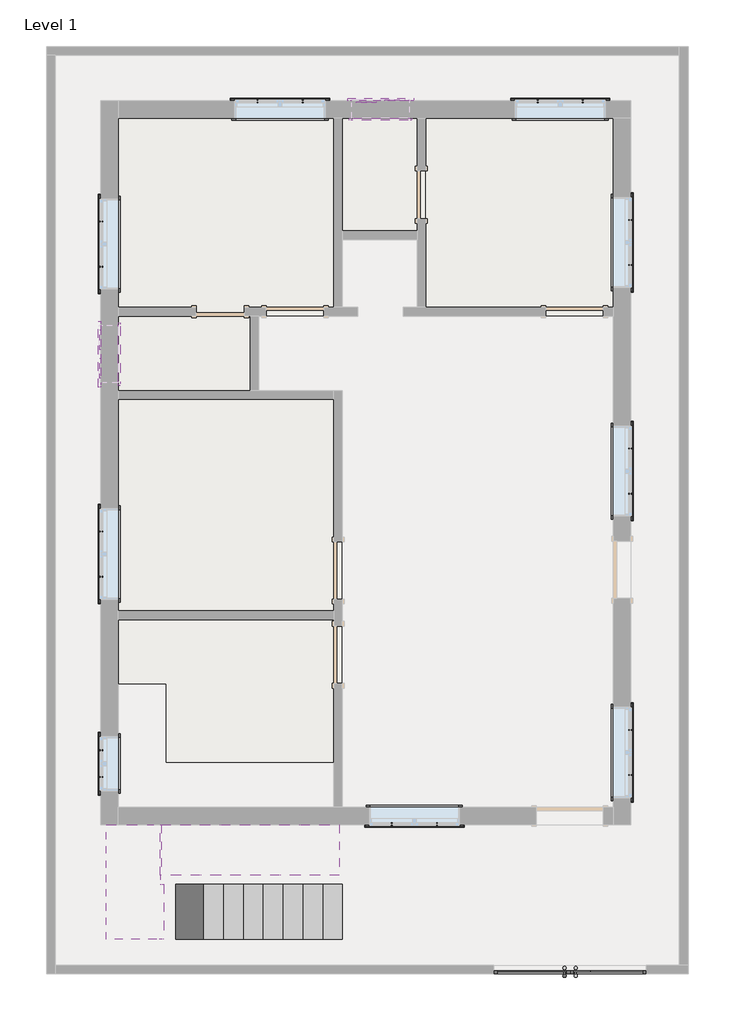
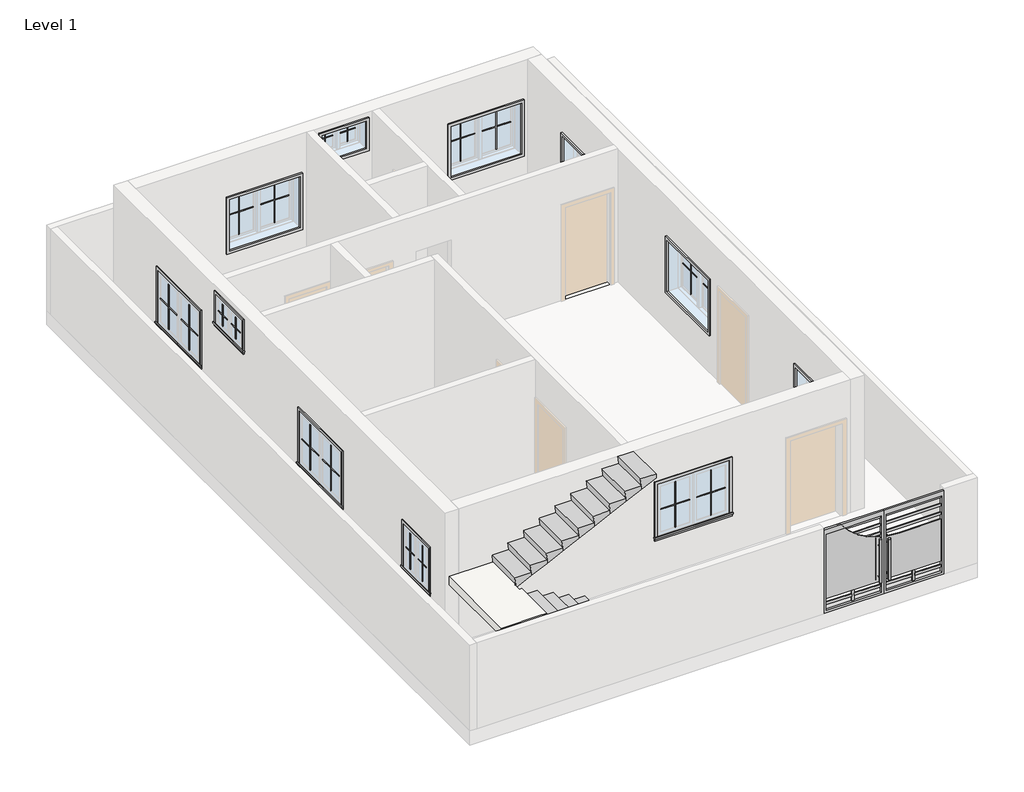
# One storey, part 2 of 2: 45 proxies, 3 slabs, 2 stair flights.
"""IFC4 building model written with IfcOpenShell, lengths in millimetres."""

from ifc_helpers import new_model, si_unit, origin, origin_with_axes, place, context, project, spatial, polyline, outline, extrude, faceted_brep, transform, mapped, element, save
from components import generic_models_9a79fa98, muntin_pattern_2x2_muntin_pattern_2x2_b3fe6957, muntin_pattern_2x2_muntin_pattern_2x2_3e0ecaf2, muntin_pattern_2x2_muntin_pattern_2x2_27d56209, muntin_pattern_2x2_muntin_pattern_2x2_bc89accc, muntin_pattern_2x2_muntin_pattern_2x2_1fe271a4, muntin_pattern_2x2_muntin_pattern_2x2_11ff06db, trim_window_exterior_flat_with_sill_41619996, trim_window_exterior_flat_with_sill_40e754a6, trim_window_exterior_flat_with_sill_f4abd27b, trim_window_interior_flat_picture_frame_51c85655, trim_window_interior_flat_picture_frame_6592d821, trim_window_interior_flat_picture_frame_286514af

model = new_model("IFC4")

# Units and contexts
model_context = context("Model", 3, world=origin())
ifc_project = project(units=[si_unit("LENGTHUNIT", "METRE", prefix="MILLI")], contexts=[model_context])

# Site, building, storey
site = spatial("IfcSite", under=ifc_project)
building = spatial("IfcBuilding", under=site)
storey = spatial("IfcBuildingStorey", under=building, Name="Level 1", Elevation=0.0)

# Proxies
placement = place(None, origin())
generic_models_shape = generic_models_9a79fa98(model_context)
element("IfcBuildingElementProxy", 1, Name="Generic Models", at=placement, inside=storey, context=model_context, shape_type="MappedRepresentation", body=[
    mapped(generic_models_shape, transform((-1347.3285282, -7397.4703663, 0.0), x_axis=(1.0, 0.0, 0.0), y_axis=(0.0, 1.0, 0.0), z_axis=(0.0, 0.0, 1.0))),
])
muntin_pattern_2x2_muntin_pattern_2x2_shape = muntin_pattern_2x2_muntin_pattern_2x2_b3fe6957(model_context)
element("IfcBuildingElementProxy", 2, Name="Muntin Pattern_2x2 : Muntin Pattern_2x2", ObjectType="Muntin Pattern_2x2 : Muntin Pattern_2x2", at=placement, inside=storey, context=model_context, shape_type="MappedRepresentation", body=[
    mapped(muntin_pattern_2x2_muntin_pattern_2x2_shape, transform((-8839.6634077, -4303.4328663, 984.25), x_axis=(0.0, 1.0, 0.0), y_axis=(-1.0, 0.0, 0.0), z_axis=(0.0, 0.0, 1.0))),
])
muntin_pattern_2x2_muntin_pattern_2x2_2_shape = muntin_pattern_2x2_muntin_pattern_2x2_3e0ecaf2(model_context)
element("IfcBuildingElementProxy", 3, Name="Muntin Pattern_2x2 : Muntin Pattern_2x2", ObjectType="Muntin Pattern_2x2 : Muntin Pattern_2x2", at=placement, inside=storey, context=model_context, shape_type="MappedRepresentation", body=[
    mapped(muntin_pattern_2x2_muntin_pattern_2x2_2_shape, transform((-8839.6634077, -3874.8078663, 984.25), x_axis=(0.0, -1.0, 0.0), y_axis=(1.0, 0.0, 0.0), z_axis=(0.0, 0.0, 1.0))),
])
muntin_pattern_2x2_muntin_pattern_2x2_3_shape = muntin_pattern_2x2_muntin_pattern_2x2_27d56209(model_context)
element("IfcBuildingElementProxy", 4, Name="Muntin Pattern_2x2 : Muntin Pattern_2x2", ObjectType="Muntin Pattern_2x2 : Muntin Pattern_2x2", at=placement, inside=storey, context=model_context, shape_type="MappedRepresentation", body=[
    mapped(muntin_pattern_2x2_muntin_pattern_2x2_3_shape, transform((-8839.6634077, 2226.7657273, 2203.45), x_axis=(0.0, 1.0, 0.0), y_axis=(-1.0, 0.0, 0.0), z_axis=(0.0, 0.0, 1.0))),
])
element("IfcBuildingElementProxy", 5, Name="Muntin Pattern_2x2 : Muntin Pattern_2x2", ObjectType="Muntin Pattern_2x2 : Muntin Pattern_2x2", at=placement, inside=storey, context=model_context, shape_type="MappedRepresentation", body=[
    mapped(muntin_pattern_2x2_muntin_pattern_2x2_3_shape, transform((-4603.9220229, 6494.5392844, 2203.45), x_axis=(1.0, 0.0, 0.0), y_axis=(0.0, 1.0, 0.0), z_axis=(0.0, 0.0, 1.0))),
])
muntin_pattern_2x2_muntin_pattern_2x2_4_shape = muntin_pattern_2x2_muntin_pattern_2x2_bc89accc(model_context)
element("IfcBuildingElementProxy", 6, Name="Muntin Pattern_2x2 : Muntin Pattern_2x2", ObjectType="Muntin Pattern_2x2 : Muntin Pattern_2x2", at=placement, inside=storey, context=model_context, shape_type="MappedRepresentation", body=[
    mapped(muntin_pattern_2x2_muntin_pattern_2x2_4_shape, transform((-8839.6634077, 2680.7907273, 2203.45), x_axis=(0.0, -1.0, 0.0), y_axis=(1.0, 0.0, 0.0), z_axis=(0.0, 0.0, 1.0))),
])
element("IfcBuildingElementProxy", 7, Name="Muntin Pattern_2x2 : Muntin Pattern_2x2", ObjectType="Muntin Pattern_2x2 : Muntin Pattern_2x2", at=placement, inside=storey, context=model_context, shape_type="MappedRepresentation", body=[
    mapped(muntin_pattern_2x2_muntin_pattern_2x2_4_shape, transform((-4149.8970229, 6494.5392844, 2203.45), x_axis=(-1.0, 0.0, 0.0), y_axis=(0.0, -1.0, 0.0), z_axis=(0.0, 0.0, 1.0))),
])
muntin_pattern_2x2_muntin_pattern_2x2_5_shape = muntin_pattern_2x2_muntin_pattern_2x2_1fe271a4(model_context)
element("IfcBuildingElementProxy", 8, Name="Muntin Pattern_2x2 : Muntin Pattern_2x2", ObjectType="Muntin Pattern_2x2 : Muntin Pattern_2x2", at=placement, inside=storey, context=model_context, shape_type="MappedRepresentation", body=[
    mapped(muntin_pattern_2x2_muntin_pattern_2x2_5_shape, transform((-385.3035282, -3550.9578663, 984.25), x_axis=(0.0, -1.0, 0.0), y_axis=(1.0, 0.0, 0.0), z_axis=(0.0, 0.0, 1.0))),
])
element("IfcBuildingElementProxy", 9, Name="Muntin Pattern_2x2 : Muntin Pattern_2x2", ObjectType="Muntin Pattern_2x2 : Muntin Pattern_2x2", at=placement, inside=storey, context=model_context, shape_type="MappedRepresentation", body=[
    mapped(muntin_pattern_2x2_muntin_pattern_2x2_5_shape, transform((-385.3035282, 944.8421337, 984.25), x_axis=(0.0, -1.0, 0.0), y_axis=(1.0, 0.0, 0.0), z_axis=(0.0, 0.0, 1.0))),
])
element("IfcBuildingElementProxy", 10, Name="Muntin Pattern_2x2 : Muntin Pattern_2x2", ObjectType="Muntin Pattern_2x2 : Muntin Pattern_2x2", at=placement, inside=storey, context=model_context, shape_type="MappedRepresentation", body=[
    mapped(muntin_pattern_2x2_muntin_pattern_2x2_5_shape, transform((-385.3035282, 4597.1928819, 984.25), x_axis=(0.0, -1.0, 0.0), y_axis=(1.0, 0.0, 0.0), z_axis=(0.0, 0.0, 1.0))),
])
element("IfcBuildingElementProxy", 11, Name="Muntin Pattern_2x2 : Muntin Pattern_2x2", ObjectType="Muntin Pattern_2x2 : Muntin Pattern_2x2", at=placement, inside=storey, context=model_context, shape_type="MappedRepresentation", body=[
    mapped(muntin_pattern_2x2_muntin_pattern_2x2_5_shape, transform((-1866.4410282, 6494.5392844, 984.25), x_axis=(1.0, 0.0, 0.0), y_axis=(0.0, 1.0, 0.0), z_axis=(0.0, 0.0, 1.0))),
])
element("IfcBuildingElementProxy", 12, Name="Muntin Pattern_2x2 : Muntin Pattern_2x2", ObjectType="Muntin Pattern_2x2 : Muntin Pattern_2x2", at=placement, inside=storey, context=model_context, shape_type="MappedRepresentation", body=[
    mapped(muntin_pattern_2x2_muntin_pattern_2x2_5_shape, transform((-6342.5074828, 6494.5392844, 984.25), x_axis=(1.0, 0.0, 0.0), y_axis=(0.0, 1.0, 0.0), z_axis=(0.0, 0.0, 1.0))),
])
element("IfcBuildingElementProxy", 13, Name="Muntin Pattern_2x2 : Muntin Pattern_2x2", ObjectType="Muntin Pattern_2x2 : Muntin Pattern_2x2", at=placement, inside=storey, context=model_context, shape_type="MappedRepresentation", body=[
    mapped(muntin_pattern_2x2_muntin_pattern_2x2_5_shape, transform((-8839.6634077, 3851.0678819, 984.25), x_axis=(0.0, 1.0, 0.0), y_axis=(-1.0, 0.0, 0.0), z_axis=(0.0, 0.0, 1.0))),
])
element("IfcBuildingElementProxy", 14, Name="Muntin Pattern_2x2 : Muntin Pattern_2x2", ObjectType="Muntin Pattern_2x2 : Muntin Pattern_2x2", at=placement, inside=storey, context=model_context, shape_type="MappedRepresentation", body=[
    mapped(muntin_pattern_2x2_muntin_pattern_2x2_5_shape, transform((-8839.6634077, -1101.0873314, 984.25), x_axis=(0.0, 1.0, 0.0), y_axis=(-1.0, 0.0, 0.0), z_axis=(0.0, 0.0, 1.0))),
])
element("IfcBuildingElementProxy", 15, Name="Muntin Pattern_2x2 : Muntin Pattern_2x2", ObjectType="Muntin Pattern_2x2 : Muntin Pattern_2x2", at=placement, inside=storey, context=model_context, shape_type="MappedRepresentation", body=[
    mapped(muntin_pattern_2x2_muntin_pattern_2x2_5_shape, transform((-3475.4824828, -5057.4953663, 984.25), x_axis=(-1.0, 0.0, 0.0), y_axis=(0.0, -1.0, 0.0), z_axis=(0.0, 0.0, 1.0))),
])
muntin_pattern_2x2_muntin_pattern_2x2_6_shape = muntin_pattern_2x2_muntin_pattern_2x2_11ff06db(model_context)
element("IfcBuildingElementProxy", 16, Name="Muntin Pattern_2x2 : Muntin Pattern_2x2", ObjectType="Muntin Pattern_2x2 : Muntin Pattern_2x2", at=placement, inside=storey, context=model_context, shape_type="MappedRepresentation", body=[
    mapped(muntin_pattern_2x2_muntin_pattern_2x2_6_shape, transform((-385.3035282, -4271.6828663, 984.25), x_axis=(0.0, 1.0, 0.0), y_axis=(-1.0, 0.0, 0.0), z_axis=(0.0, 0.0, 1.0))),
])
element("IfcBuildingElementProxy", 17, Name="Muntin Pattern_2x2 : Muntin Pattern_2x2", ObjectType="Muntin Pattern_2x2 : Muntin Pattern_2x2", at=placement, inside=storey, context=model_context, shape_type="MappedRepresentation", body=[
    mapped(muntin_pattern_2x2_muntin_pattern_2x2_6_shape, transform((-385.3035282, 224.1171337, 984.25), x_axis=(0.0, 1.0, 0.0), y_axis=(-1.0, 0.0, 0.0), z_axis=(0.0, 0.0, 1.0))),
])
element("IfcBuildingElementProxy", 18, Name="Muntin Pattern_2x2 : Muntin Pattern_2x2", ObjectType="Muntin Pattern_2x2 : Muntin Pattern_2x2", at=placement, inside=storey, context=model_context, shape_type="MappedRepresentation", body=[
    mapped(muntin_pattern_2x2_muntin_pattern_2x2_6_shape, transform((-385.3035282, 3876.4678819, 984.25), x_axis=(0.0, 1.0, 0.0), y_axis=(-1.0, 0.0, 0.0), z_axis=(0.0, 0.0, 1.0))),
])
element("IfcBuildingElementProxy", 19, Name="Muntin Pattern_2x2 : Muntin Pattern_2x2", ObjectType="Muntin Pattern_2x2 : Muntin Pattern_2x2", at=placement, inside=storey, context=model_context, shape_type="MappedRepresentation", body=[
    mapped(muntin_pattern_2x2_muntin_pattern_2x2_6_shape, transform((-1145.7160282, 6494.5392844, 984.25), x_axis=(-1.0, 0.0, 0.0), y_axis=(0.0, -1.0, 0.0), z_axis=(0.0, 0.0, 1.0))),
])
element("IfcBuildingElementProxy", 20, Name="Muntin Pattern_2x2 : Muntin Pattern_2x2", ObjectType="Muntin Pattern_2x2 : Muntin Pattern_2x2", at=placement, inside=storey, context=model_context, shape_type="MappedRepresentation", body=[
    mapped(muntin_pattern_2x2_muntin_pattern_2x2_6_shape, transform((-5621.7824828, 6494.5392844, 984.25), x_axis=(-1.0, 0.0, 0.0), y_axis=(0.0, -1.0, 0.0), z_axis=(0.0, 0.0, 1.0))),
])
element("IfcBuildingElementProxy", 21, Name="Muntin Pattern_2x2 : Muntin Pattern_2x2", ObjectType="Muntin Pattern_2x2 : Muntin Pattern_2x2", at=placement, inside=storey, context=model_context, shape_type="MappedRepresentation", body=[
    mapped(muntin_pattern_2x2_muntin_pattern_2x2_6_shape, transform((-8839.6634077, 4571.7928819, 984.25), x_axis=(0.0, -1.0, 0.0), y_axis=(1.0, 0.0, 0.0), z_axis=(0.0, 0.0, 1.0))),
])
element("IfcBuildingElementProxy", 22, Name="Muntin Pattern_2x2 : Muntin Pattern_2x2", ObjectType="Muntin Pattern_2x2 : Muntin Pattern_2x2", at=placement, inside=storey, context=model_context, shape_type="MappedRepresentation", body=[
    mapped(muntin_pattern_2x2_muntin_pattern_2x2_6_shape, transform((-8839.6634077, -380.3623314, 984.25), x_axis=(0.0, -1.0, 0.0), y_axis=(1.0, 0.0, 0.0), z_axis=(0.0, 0.0, 1.0))),
])
element("IfcBuildingElementProxy", 23, Name="Muntin Pattern_2x2 : Muntin Pattern_2x2", ObjectType="Muntin Pattern_2x2 : Muntin Pattern_2x2", at=placement, inside=storey, context=model_context, shape_type="MappedRepresentation", body=[
    mapped(muntin_pattern_2x2_muntin_pattern_2x2_6_shape, transform((-4196.2074828, -5057.4953663, 984.25), x_axis=(1.0, 0.0, 0.0), y_axis=(0.0, 1.0, 0.0), z_axis=(0.0, 0.0, 1.0))),
])
trim_window_exterior_flat_with_sill_shape = trim_window_exterior_flat_with_sill_41619996(model_context)
element("IfcBuildingElementProxy", 24, Name="Trim-Window-Exterior-Flat : with Sill", ObjectType="Trim-Window-Exterior-Flat : with Sill", at=placement, inside=storey, context=model_context, shape_type="MappedRepresentation", body=[
    mapped(trim_window_exterior_flat_with_sill_shape, transform((-8849.1884077, -4089.1203663, 1828.8), x_axis=(0.0, -1.0, 0.0), y_axis=(0.0, 0.0, 1.0), z_axis=(-1.0, 0.0, 0.0))),
])
trim_window_exterior_flat_with_sill_2_shape = trim_window_exterior_flat_with_sill_40e754a6(model_context)
element("IfcBuildingElementProxy", 25, Name="Trim-Window-Exterior-Flat : with Sill", ObjectType="Trim-Window-Exterior-Flat : with Sill", at=placement, inside=storey, context=model_context, shape_type="MappedRepresentation", body=[
    mapped(trim_window_exterior_flat_with_sill_2_shape, transform((-8849.1884077, 2453.7782273, 2743.2), x_axis=(0.0, -1.0, 0.0), y_axis=(0.0, 0.0, 1.0), z_axis=(-1.0, 0.0, 0.0))),
])
element("IfcBuildingElementProxy", 26, Name="Trim-Window-Exterior-Flat : with Sill", ObjectType="Trim-Window-Exterior-Flat : with Sill", at=placement, inside=storey, context=model_context, shape_type="MappedRepresentation", body=[
    mapped(trim_window_exterior_flat_with_sill_2_shape, transform((-4376.9095229, 6504.0642844, 2743.2), x_axis=(-1.0, 0.0, 0.0), y_axis=(0.0, 0.0, 1.0), z_axis=(0.0, 1.0, 0.0))),
])
trim_window_exterior_flat_with_sill_3_shape = trim_window_exterior_flat_with_sill_f4abd27b(model_context)
element("IfcBuildingElementProxy", 27, Name="Trim-Window-Exterior-Flat : with Sill", ObjectType="Trim-Window-Exterior-Flat : with Sill", at=placement, inside=storey, context=model_context, shape_type="MappedRepresentation", body=[
    mapped(trim_window_exterior_flat_with_sill_3_shape, transform((-375.7785282, -3911.3203663, 2032.0), x_axis=(0.0, 1.0, 0.0), y_axis=(0.0, 0.0, 1.0), z_axis=(1.0, 0.0, 0.0))),
])
element("IfcBuildingElementProxy", 28, Name="Trim-Window-Exterior-Flat : with Sill", ObjectType="Trim-Window-Exterior-Flat : with Sill", at=placement, inside=storey, context=model_context, shape_type="MappedRepresentation", body=[
    mapped(trim_window_exterior_flat_with_sill_3_shape, transform((-375.7785282, 584.4796337, 2032.0), x_axis=(0.0, 1.0, 0.0), y_axis=(0.0, 0.0, 1.0), z_axis=(1.0, 0.0, 0.0))),
])
element("IfcBuildingElementProxy", 29, Name="Trim-Window-Exterior-Flat : with Sill", ObjectType="Trim-Window-Exterior-Flat : with Sill", at=placement, inside=storey, context=model_context, shape_type="MappedRepresentation", body=[
    mapped(trim_window_exterior_flat_with_sill_3_shape, transform((-375.7785282, 4236.8303819, 2032.0), x_axis=(0.0, 1.0, 0.0), y_axis=(0.0, 0.0, 1.0), z_axis=(1.0, 0.0, 0.0))),
])
element("IfcBuildingElementProxy", 30, Name="Trim-Window-Exterior-Flat : with Sill", ObjectType="Trim-Window-Exterior-Flat : with Sill", at=placement, inside=storey, context=model_context, shape_type="MappedRepresentation", body=[
    mapped(trim_window_exterior_flat_with_sill_3_shape, transform((-1506.0785282, 6504.0642844, 2032.0), x_axis=(-1.0, 0.0, 0.0), y_axis=(0.0, 0.0, 1.0), z_axis=(0.0, 1.0, 0.0))),
])
element("IfcBuildingElementProxy", 31, Name="Trim-Window-Exterior-Flat : with Sill", ObjectType="Trim-Window-Exterior-Flat : with Sill", at=placement, inside=storey, context=model_context, shape_type="MappedRepresentation", body=[
    mapped(trim_window_exterior_flat_with_sill_3_shape, transform((-5982.1449828, 6504.0642844, 2032.0), x_axis=(-1.0, 0.0, 0.0), y_axis=(0.0, 0.0, 1.0), z_axis=(0.0, 1.0, 0.0))),
])
element("IfcBuildingElementProxy", 32, Name="Trim-Window-Exterior-Flat : with Sill", ObjectType="Trim-Window-Exterior-Flat : with Sill", at=placement, inside=storey, context=model_context, shape_type="MappedRepresentation", body=[
    mapped(trim_window_exterior_flat_with_sill_3_shape, transform((-8849.1884077, 4211.4303819, 2032.0), x_axis=(0.0, -1.0, 0.0), y_axis=(0.0, 0.0, 1.0), z_axis=(-1.0, 0.0, 0.0))),
])
element("IfcBuildingElementProxy", 33, Name="Trim-Window-Exterior-Flat : with Sill", ObjectType="Trim-Window-Exterior-Flat : with Sill", at=placement, inside=storey, context=model_context, shape_type="MappedRepresentation", body=[
    mapped(trim_window_exterior_flat_with_sill_3_shape, transform((-8849.1884077, -740.7248314, 2032.0), x_axis=(0.0, -1.0, 0.0), y_axis=(0.0, 0.0, 1.0), z_axis=(-1.0, 0.0, 0.0))),
])
element("IfcBuildingElementProxy", 34, Name="Trim-Window-Exterior-Flat : with Sill", ObjectType="Trim-Window-Exterior-Flat : with Sill", at=placement, inside=storey, context=model_context, shape_type="MappedRepresentation", body=[
    mapped(trim_window_exterior_flat_with_sill_3_shape, transform((-3835.8449828, -5067.0203663, 2032.0), x_axis=(1.0, 0.0, 0.0), y_axis=(0.0, 0.0, 1.0), z_axis=(0.0, -1.0, 0.0))),
])
trim_window_interior_flat_picture_frame_shape = trim_window_interior_flat_picture_frame_51c85655(model_context)
element("IfcBuildingElementProxy", 35, Name="Trim-Window-Interior-Flat : Picture Frame", ObjectType="Trim-Window-Interior-Flat : Picture Frame", at=placement, inside=storey, context=model_context, shape_type="MappedRepresentation", body=[
    mapped(trim_window_interior_flat_picture_frame_shape, transform((-8569.7884077, -4089.1203663, 1828.8), x_axis=(0.0, 1.0, 0.0), y_axis=(0.0, 0.0, 1.0), z_axis=(1.0, 0.0, 0.0))),
])
trim_window_interior_flat_picture_frame_2_shape = trim_window_interior_flat_picture_frame_6592d821(model_context)
element("IfcBuildingElementProxy", 36, Name="Trim-Window-Interior-Flat : Picture Frame", ObjectType="Trim-Window-Interior-Flat : Picture Frame", at=placement, inside=storey, context=model_context, shape_type="MappedRepresentation", body=[
    mapped(trim_window_interior_flat_picture_frame_2_shape, transform((-8569.7884077, 2453.7782273, 2743.2), x_axis=(0.0, 1.0, 0.0), y_axis=(0.0, 0.0, 1.0), z_axis=(1.0, 0.0, 0.0))),
])
element("IfcBuildingElementProxy", 37, Name="Trim-Window-Interior-Flat : Picture Frame", ObjectType="Trim-Window-Interior-Flat : Picture Frame", at=placement, inside=storey, context=model_context, shape_type="MappedRepresentation", body=[
    mapped(trim_window_interior_flat_picture_frame_2_shape, transform((-4376.9095229, 6224.6642844, 2743.2), x_axis=(1.0, 0.0, 0.0), y_axis=(0.0, 0.0, 1.0), z_axis=(0.0, -1.0, 0.0))),
])
trim_window_interior_flat_picture_frame_3_shape = trim_window_interior_flat_picture_frame_286514af(model_context)
element("IfcBuildingElementProxy", 38, Name="Trim-Window-Interior-Flat : Picture Frame", ObjectType="Trim-Window-Interior-Flat : Picture Frame", at=placement, inside=storey, context=model_context, shape_type="MappedRepresentation", body=[
    mapped(trim_window_interior_flat_picture_frame_3_shape, transform((-655.1785282, -3911.3203663, 2032.0), x_axis=(0.0, -1.0, 0.0), y_axis=(0.0, 0.0, 1.0), z_axis=(-1.0, 0.0, 0.0))),
])
element("IfcBuildingElementProxy", 39, Name="Trim-Window-Interior-Flat : Picture Frame", ObjectType="Trim-Window-Interior-Flat : Picture Frame", at=placement, inside=storey, context=model_context, shape_type="MappedRepresentation", body=[
    mapped(trim_window_interior_flat_picture_frame_3_shape, transform((-655.1785282, 584.4796337, 2032.0), x_axis=(0.0, -1.0, 0.0), y_axis=(0.0, 0.0, 1.0), z_axis=(-1.0, 0.0, 0.0))),
])
element("IfcBuildingElementProxy", 40, Name="Trim-Window-Interior-Flat : Picture Frame", ObjectType="Trim-Window-Interior-Flat : Picture Frame", at=placement, inside=storey, context=model_context, shape_type="MappedRepresentation", body=[
    mapped(trim_window_interior_flat_picture_frame_3_shape, transform((-655.1785282, 4236.8303819, 2032.0), x_axis=(0.0, -1.0, 0.0), y_axis=(0.0, 0.0, 1.0), z_axis=(-1.0, 0.0, 0.0))),
])
element("IfcBuildingElementProxy", 41, Name="Trim-Window-Interior-Flat : Picture Frame", ObjectType="Trim-Window-Interior-Flat : Picture Frame", at=placement, inside=storey, context=model_context, shape_type="MappedRepresentation", body=[
    mapped(trim_window_interior_flat_picture_frame_3_shape, transform((-1506.0785282, 6224.6642844, 2032.0), x_axis=(1.0, 0.0, 0.0), y_axis=(0.0, 0.0, 1.0), z_axis=(0.0, -1.0, 0.0))),
])
element("IfcBuildingElementProxy", 42, Name="Trim-Window-Interior-Flat : Picture Frame", ObjectType="Trim-Window-Interior-Flat : Picture Frame", at=placement, inside=storey, context=model_context, shape_type="MappedRepresentation", body=[
    mapped(trim_window_interior_flat_picture_frame_3_shape, transform((-5982.1449828, 6224.6642844, 2032.0), x_axis=(1.0, 0.0, 0.0), y_axis=(0.0, 0.0, 1.0), z_axis=(0.0, -1.0, 0.0))),
])
element("IfcBuildingElementProxy", 43, Name="Trim-Window-Interior-Flat : Picture Frame", ObjectType="Trim-Window-Interior-Flat : Picture Frame", at=placement, inside=storey, context=model_context, shape_type="MappedRepresentation", body=[
    mapped(trim_window_interior_flat_picture_frame_3_shape, transform((-8569.7884077, 4211.4303819, 2032.0), x_axis=(0.0, 1.0, 0.0), y_axis=(0.0, 0.0, 1.0), z_axis=(1.0, 0.0, 0.0))),
])
element("IfcBuildingElementProxy", 44, Name="Trim-Window-Interior-Flat : Picture Frame", ObjectType="Trim-Window-Interior-Flat : Picture Frame", at=placement, inside=storey, context=model_context, shape_type="MappedRepresentation", body=[
    mapped(trim_window_interior_flat_picture_frame_3_shape, transform((-8569.7884077, -740.7248314, 2032.0), x_axis=(0.0, 1.0, 0.0), y_axis=(0.0, 0.0, 1.0), z_axis=(1.0, 0.0, 0.0))),
])
element("IfcBuildingElementProxy", 45, Name="Trim-Window-Interior-Flat : Picture Frame", ObjectType="Trim-Window-Interior-Flat : Picture Frame", at=placement, inside=storey, context=model_context, shape_type="MappedRepresentation", body=[
    mapped(trim_window_interior_flat_picture_frame_3_shape, transform((-3835.8449828, -4787.6203663, 2032.0), x_axis=(-1.0, 0.0, 0.0), y_axis=(0.0, 0.0, 1.0), z_axis=(0.0, 1.0, 0.0))),
])

# Slabs
element("IfcSlab", 46, ObjectType="7\" Thickness", at=placement, inside=storey, context=model_context, shape_type="Brep", body=[
    faceted_brep([(-7896.6884077, -6018.2039507, 1524.0), (-7896.6884077, -5868.2058051, 1524.0), (-7877.6384077, -5868.2058051, 1524.0), (-7877.6384077, -5067.0203663, 1524.0), (-7896.6884077, -5067.0203663, 1524.0), (-8101.3126638, -5067.0203663, 1524.0), (-8760.2884077, -5067.0203663, 1524.0), (-8760.2884077, -6894.0922127, 1524.0), (-7955.5707267, -6894.0922127, 1524.0), (-7842.6949828, -6894.0922127, 1524.0), (-7842.6949828, -6018.2039507, 1524.0), (-7861.7449828, -6018.2039507, 1371.6), (-7861.7449828, -6894.0922127, 1371.6), (-7861.7449828, -6894.0922127, 1301.1636429), (-7861.7449828, -6018.2039507, 1301.1636429), (-7955.5707267, -6018.2039507, 1346.2), (-7896.6884077, -6018.2039507, 1346.2), (-7896.6884077, -5868.2058051, 1346.2), (-7896.6884077, -5868.2058051, 1444.4196429), (-7877.6384077, -5868.2058051, 1453.5636429), (-7877.6384077, -5067.0203663, 1453.5636429), (-7896.6884077, -5067.0203663, 1444.4196429), (-8101.3126638, -5067.0203663, 1346.2), (-8760.2884077, -5067.0203663, 1346.2), (-8760.2884077, -6894.0922127, 1346.2), (-7955.5707267, -6894.0922127, 1346.2), (-8101.3126638, -5868.2058051, 1346.2)], [[[0, 1, 2, 3, 4, 5, 6, 7, 8, 9, 10]], [[11, 12, 13, 14]], [[0, 10, 11, 14, 15, 16]], [[1, 0, 16, 17, 18]], [[2, 1, 18, 19]], [[3, 2, 19, 20]], [[4, 3, 20, 21]], [[4, 21, 22, 23, 6, 5]], [[7, 6, 23, 24]], [[12, 9, 8, 7, 24, 25, 13]], [[10, 9, 12, 11]], [[26, 17, 16, 15, 25, 24, 23, 22]], [[17, 26, 18]], [[25, 15, 14, 13]], [[26, 22, 21, 20, 19, 18]]]),
])
element("IfcSlab", 47, ObjectType="BED ROOM FLOOR", at=placement, inside=storey, context=model_context, shape_type="SweptSolid", body=[
    extrude(outline(polyline([(-4985.1949828, -4787.6203663), (-8569.7884077, -4787.6203663), (-8569.7884077, -1788.4748314), (-4985.1949828, -1788.4748314), (-4985.1949828, -4787.6203663)])), origin_with_axes(), (0.0, 0.0, 1.0), 50.8),
    extrude(outline(polyline([(-4985.1949828, -1672.5465885), (-8569.7884077, -1672.5465885), (-8569.7884077, 1731.1760727), (-4985.1949828, 1731.1760727), (-4985.1949828, -1672.5465885)])), origin_with_axes(), (0.0, 0.0, 1.0), 50.8),
    extrude(outline(polyline([(-8569.7884077, 6224.6642844), (-5124.8949828, 6224.6642844), (-5124.8949828, 3062.0803819), (-8569.7884077, 3062.0803819), (-8569.7884077, 6224.6642844)])), origin_with_axes(), (0.0, 0.0, 1.0), 50.8),
    extrude(outline(polyline([(-655.1785282, 6224.6642844), (-655.1785282, 3062.0803819), (-3654.3240631, 3062.0803819), (-3654.3240631, 6224.6642844), (-655.1785282, 6224.6642844)])), origin_with_axes(), (0.0, 0.0, 1.0), 50.8),
])
element("IfcSlab", 48, ObjectType="TOILET FLOORING", at=placement, inside=storey, context=model_context, shape_type="SweptSolid", body=[
    extrude(outline(polyline([(-6432.0275348, 3201.7803819), (-6432.0275348, 1842.4631791), (-8569.7884077, 1842.4631791), (-8569.7884077, 3201.7803819), (-6432.0275348, 3201.7803819)])), origin_with_axes(), (0.0, 0.0, 1.0), 50.8),
    extrude(outline(polyline([(-3654.3240631, 6224.6642844), (-3654.3240631, 4397.592438), (-4985.1949828, 4397.592438), (-4985.1949828, 6224.6642844), (-3654.3240631, 6224.6642844)])), origin_with_axes(), (0.0, 0.0, 1.0), 50.8),
])

# Stair flights
element("IfcStairFlight", 49, ObjectType="3/4\" Nosing", at=placement, inside=storey, context=model_context, shape_type="Brep", body=[
    faceted_brep([(-4985.1949828, -6894.0922127, 152.4), (-4985.1949828, -6018.2039507, 152.4), (-5321.7449828, -6018.2039507, 152.4), (-5321.7449828, -6894.0922127, 152.4), (-5321.7449828, -6894.0922127, 81.9636429), (-5150.9873934, -6894.0922127, 0.0), (-5004.2449828, -6894.0922127, 0.0), (-5004.2449828, -6018.2039507, 0.0), (-5150.9873934, -6018.2039507, 0.0), (-5321.7449828, -6018.2039507, 81.9636429), (-5302.6949828, -6894.0922127, 304.8), (-5302.6949828, -6018.2039507, 304.8), (-5639.2449828, -6018.2039507, 304.8), (-5639.2449828, -6894.0922127, 304.8), (-5639.2449828, -6894.0922127, 234.3636429), (-5639.2449828, -6018.2039507, 234.3636429), (-5620.1949828, -6894.0922127, 457.2), (-5620.1949828, -6018.2039507, 457.2), (-5956.7449828, -6018.2039507, 457.2), (-5956.7449828, -6894.0922127, 457.2), (-5956.7449828, -6894.0922127, 386.7636429), (-5956.7449828, -6018.2039507, 386.7636429), (-5937.6949828, -6894.0922127, 609.6), (-5937.6949828, -6018.2039507, 609.6), (-6274.2449828, -6018.2039507, 609.6), (-6274.2449828, -6894.0922127, 609.6), (-6274.2449828, -6894.0922127, 539.1636429), (-6274.2449828, -6018.2039507, 539.1636429), (-6255.1949828, -6894.0922127, 762.0), (-6255.1949828, -6018.2039507, 762.0), (-6591.7449828, -6018.2039507, 762.0), (-6591.7449828, -6894.0922127, 762.0), (-6591.7449828, -6894.0922127, 691.5636429), (-6591.7449828, -6018.2039507, 691.5636429), (-6572.6949828, -6894.0922127, 914.4), (-6572.6949828, -6018.2039507, 914.4), (-6909.2449828, -6018.2039507, 914.4), (-6909.2449828, -6894.0922127, 914.4), (-6909.2449828, -6894.0922127, 843.9636429), (-6909.2449828, -6018.2039507, 843.9636429), (-6890.1949828, -6894.0922127, 1066.8), (-6890.1949828, -6018.2039507, 1066.8), (-7226.7449828, -6018.2039507, 1066.8), (-7226.7449828, -6894.0922127, 1066.8), (-7226.7449828, -6894.0922127, 996.3636429), (-7226.7449828, -6018.2039507, 996.3636429), (-7207.6949828, -6894.0922127, 1219.2), (-7207.6949828, -6018.2039507, 1219.2), (-7544.2449828, -6018.2039507, 1219.2), (-7544.2449828, -6894.0922127, 1219.2), (-7544.2449828, -6894.0922127, 1148.7636429), (-7544.2449828, -6018.2039507, 1148.7636429), (-7861.7449828, -6894.0922127, 1371.6), (-7842.6949828, -6894.0922127, 1371.6), (-7525.1949828, -6894.0922127, 1371.6), (-7525.1949828, -6018.2039507, 1371.6), (-7842.6949828, -6018.2039507, 1371.6), (-7861.7449828, -6018.2039507, 1371.6), (-7861.7449828, -6894.0922127, 1301.1636429), (-7842.6949828, -6894.0922127, 1292.0196429), (-7842.6949828, -6018.2039507, 1292.0196429), (-7861.7449828, -6018.2039507, 1301.1636429)], [[[0, 1, 2, 3]], [[0, 3, 4, 5, 6]], [[2, 1, 7, 8, 9]], [[10, 11, 12, 13]], [[10, 13, 14, 4, 3]], [[12, 11, 2, 9, 15]], [[16, 17, 18, 19]], [[16, 19, 20, 14, 13]], [[18, 17, 12, 15, 21]], [[22, 23, 24, 25]], [[22, 25, 26, 20, 19]], [[24, 23, 18, 21, 27]], [[28, 29, 30, 31]], [[28, 31, 32, 26, 25]], [[30, 29, 24, 27, 33]], [[34, 35, 36, 37]], [[34, 37, 38, 32, 31]], [[36, 35, 30, 33, 39]], [[40, 41, 42, 43]], [[40, 43, 44, 38, 37]], [[42, 41, 36, 39, 45]], [[46, 47, 48, 49]], [[46, 49, 50, 44, 43]], [[48, 47, 42, 45, 51]], [[52, 53, 54, 55, 56, 57]], [[53, 52, 58, 59]], [[54, 53, 59, 50, 49]], [[56, 55, 48, 51, 60]], [[57, 56, 60, 61]], [[52, 57, 61, 58]], [[1, 0, 6, 7]], [[3, 2, 11, 10]], [[13, 12, 17, 16]], [[19, 18, 23, 22]], [[25, 24, 29, 28]], [[31, 30, 35, 34]], [[37, 36, 41, 40]], [[43, 42, 47, 46]], [[49, 48, 55, 54]], [[7, 6, 5, 8]], [[8, 5, 4, 14, 20, 26, 32, 38, 44, 50, 59, 58, 61, 60, 51, 45, 39, 33, 27, 21, 15, 9]]]),
])
element("IfcStairFlight", 50, ObjectType="3/4\" Nosing", at=placement, inside=storey, context=model_context, shape_type="Brep", body=[
    faceted_brep([(-7896.6884077, -5067.0203663, 1676.4), (-7896.6884077, -5868.2058051, 1676.4), (-7560.1384077, -5868.2058051, 1676.4), (-7560.1384077, -5067.0203663, 1676.4), (-7560.1384077, -5067.0203663, 1605.9636429), (-7877.6384077, -5067.0203663, 1453.5636429), (-7877.6384077, -5067.0203663, 1524.0), (-7877.6384077, -5868.2058051, 1524.0), (-7877.6384077, -5868.2058051, 1453.5636429), (-7560.1384077, -5868.2058051, 1605.9636429), (-7579.1884077, -5067.0203663, 1828.8), (-7579.1884077, -5868.2058051, 1828.8), (-7242.6384077, -5868.2058051, 1828.8), (-7242.6384077, -5067.0203663, 1828.8), (-7242.6384077, -5067.0203663, 1758.3636429), (-7242.6384077, -5868.2058051, 1758.3636429), (-7261.6884077, -5067.0203663, 1981.2), (-7261.6884077, -5868.2058051, 1981.2), (-6925.1384077, -5868.2058051, 1981.2), (-6925.1384077, -5067.0203663, 1981.2), (-6925.1384077, -5067.0203663, 1910.7636429), (-6925.1384077, -5868.2058051, 1910.7636429), (-6944.1884077, -5067.0203663, 2133.6), (-6944.1884077, -5868.2058051, 2133.6), (-6607.6384077, -5868.2058051, 2133.6), (-6607.6384077, -5067.0203663, 2133.6), (-6607.6384077, -5067.0203663, 2063.1636429), (-6607.6384077, -5868.2058051, 2063.1636429), (-6626.6884077, -5067.0203663, 2286.0), (-6626.6884077, -5868.2058051, 2286.0), (-6290.1384077, -5868.2058051, 2286.0), (-6290.1384077, -5067.0203663, 2286.0), (-6290.1384077, -5067.0203663, 2215.5636429), (-6290.1384077, -5868.2058051, 2215.5636429), (-6309.1884077, -5067.0203663, 2438.4), (-6309.1884077, -5868.2058051, 2438.4), (-5972.6384077, -5868.2058051, 2438.4), (-5972.6384077, -5067.0203663, 2438.4), (-5972.6384077, -5067.0203663, 2367.9636429), (-5972.6384077, -5868.2058051, 2367.9636429), (-5991.6884077, -5067.0203663, 2590.8), (-5991.6884077, -5868.2058051, 2590.8), (-5655.1384077, -5868.2058051, 2590.8), (-5655.1384077, -5067.0203663, 2590.8), (-5655.1384077, -5067.0203663, 2520.3636429), (-5655.1384077, -5868.2058051, 2520.3636429), (-5674.1884077, -5067.0203663, 2743.2), (-5674.1884077, -5868.2058051, 2743.2), (-5337.6384077, -5868.2058051, 2743.2), (-5337.6384077, -5067.0203663, 2743.2), (-5337.6384077, -5067.0203663, 2672.7636429), (-5337.6384077, -5868.2058051, 2672.7636429), (-5356.6884077, -5067.0203663, 2895.6), (-5356.6884077, -5868.2058051, 2895.6), (-5039.1884077, -5868.2058051, 2895.6), (-5039.1884077, -5067.0203663, 2895.6), (-5039.1884077, -5067.0203663, 2816.0196429), (-5039.1884077, -5868.2058051, 2816.0196429)], [[[0, 1, 2, 3]], [[0, 3, 4, 5, 6]], [[7, 6, 5, 8]], [[2, 1, 7, 8, 9]], [[10, 11, 12, 13]], [[10, 13, 14, 4, 3]], [[12, 11, 2, 9, 15]], [[16, 17, 18, 19]], [[16, 19, 20, 14, 13]], [[18, 17, 12, 15, 21]], [[22, 23, 24, 25]], [[22, 25, 26, 20, 19]], [[24, 23, 18, 21, 27]], [[28, 29, 30, 31]], [[28, 31, 32, 26, 25]], [[30, 29, 24, 27, 33]], [[34, 35, 36, 37]], [[34, 37, 38, 32, 31]], [[36, 35, 30, 33, 39]], [[40, 41, 42, 43]], [[40, 43, 44, 38, 37]], [[42, 41, 36, 39, 45]], [[46, 47, 48, 49]], [[46, 49, 50, 44, 43]], [[48, 47, 42, 45, 51]], [[1, 0, 6, 7]], [[11, 10, 3, 2]], [[17, 16, 13, 12]], [[23, 22, 19, 18]], [[29, 28, 25, 24]], [[35, 34, 31, 30]], [[41, 40, 37, 36]], [[47, 46, 43, 42]], [[52, 53, 54, 55]], [[52, 55, 56, 50, 49]], [[54, 53, 48, 51, 57]], [[55, 54, 57, 56]], [[53, 52, 49, 48]], [[5, 4, 14, 20, 26, 32, 38, 44, 50, 56, 57, 51, 45, 39, 33, 27, 21, 15, 9, 8]]]),
])

save(model, "model.ifc")

# Revit data of these elements
# Type
#   sheet = none
#   pipe = none
#   handal = none
#   faram = none
#   Default Elevation = 0
# Type "Muntin Pattern_2x2 : Muntin Pattern_2x2"
#   Width [instance default] = 48"
#   Thickness = 0.5"
#   Height [instance default] = 48"
#   Distance = 0.75"
#   Interior Material [instance default] = none
#   Exterior Material [instance default] = none
#   Default Elevation = 0
# Type "Trim-Window-Exterior-Flat : with Sill"
#   Trim Width = 2.25"
#   Trim Thickness_Picture Frame = 1.25"
#   Trim Thickness_with Sill = 0.75"
#   Sill Thickness = 1.25"
#   Opening Width [instance default] = 24"
#   Opening Height [instance default] = 36"
#   Default Elevation = 48"
#   Sill = yes
#   Picture Frame = no
#   Trim Material [instance default] = none
# Type "Trim-Window-Interior-Flat : Picture Frame"
#   Trim Thickness_Picture Frame = 1.25"
#   Trim Width = 2.25"
#   Trim Thickness_with Sill = 0.75"
#   Sill Thickness = 1.25"
#   Opening Width [instance default] = 24"
#   Opening Height [instance default] = 36"
#   Default Elevation = 48"
#   Sill = no
#   Picture Frame = yes
#   Trim Material [instance default] = none
# Type "BED ROOM FLOOR"
#   Assembly Code = "B1010"
#   Function = 0
#   Layers, outside or top first: 1" "BED ROOM FLOORING" (function 1); 1" no material (function 1)
# Type "TOILET FLOORING"
#   Assembly Code = "B1010"
#   Function = 0
#   Layers, outside or top first: 1" "TOILET FLOORING" (function 1); 1" no material (function 1)
# Element 1 (IfcBuildingElementProxy)
#   Phase Created = New Construction
# Elements 2, 3 (IfcBuildingElementProxy, "Muntin Pattern_2x2 : Muntin Pattern_2x2")
#   Width = 11.625"
#   Height = 30.5"
#   Interior Material = Wood - Stained
#   Exterior Material = Clad - White
#   Phase Created = New Construction
#   Materials on its faces: "Clad - White", "Wood - Stained"
# Elements 4, 5, 6, 7 (IfcBuildingElementProxy, "Muntin Pattern_2x2 : Muntin Pattern_2x2")
#   Width = 12.625"
#   Height = 18.5"
#   Interior Material = Wood - Stained
#   Exterior Material = Clad - White
#   Phase Created = New Construction
#   Materials on its faces: "Clad - White", "Wood - Stained"
# Elements 8, 9, 10, 11, 12, 13, 14, 15, 16, 17, 18, 19, 20, 21, 22, 23 (IfcBuildingElementProxy, "Muntin Pattern_2x2 : Muntin Pattern_2x2")
#   Width = 23.125"
#   Height = 38.5"
#   Interior Material = Wood - Stained
#   Exterior Material = Clad - White
#   Phase Created = New Construction
#   Materials on its faces: "Clad - White", "Wood - Stained"
# Element 24 (IfcBuildingElementProxy, "Trim-Window-Exterior-Flat : with Sill")
#   Opening Width = 34"
#   Opening Height = 36"
#   Trim Material = Clad - White
#   Phase Created = New Construction
#   Materials on its faces: "Clad - White"
# Elements 25, 26 (IfcBuildingElementProxy, "Trim-Window-Exterior-Flat : with Sill")
#   Opening Width = 36"
#   Opening Height = 24"
#   Trim Material = Clad - White
#   Phase Created = New Construction
#   Materials on its faces: "Clad - White"
# Elements 27, 28, 29, 30, 31, 32, 33, 34 (IfcBuildingElementProxy, "Trim-Window-Exterior-Flat : with Sill")
#   Opening Width = 57"
#   Opening Height = 44"
#   Trim Material = Clad - White
#   Phase Created = New Construction
#   Materials on its faces: "Clad - White"
# Element 35 (IfcBuildingElementProxy, "Trim-Window-Interior-Flat : Picture Frame")
#   Opening Width = 34"
#   Opening Height = 36"
#   Trim Material = Wood - Stained
#   Phase Created = New Construction
#   Materials on its faces: "Wood - Stained"
# Elements 36, 37 (IfcBuildingElementProxy, "Trim-Window-Interior-Flat : Picture Frame")
#   Opening Width = 36"
#   Opening Height = 24"
#   Trim Material = Wood - Stained
#   Phase Created = New Construction
#   Materials on its faces: "Wood - Stained"
# Elements 38, 39, 40, 41, 42, 43, 44, 45 (IfcBuildingElementProxy, "Trim-Window-Interior-Flat : Picture Frame")
#   Opening Width = 57"
#   Opening Height = 44"
#   Trim Material = Wood - Stained
#   Phase Created = New Construction
#   Materials on its faces: "Wood - Stained"
# Element 46 (IfcSlab, "7\" Thickness")
#   Phase Created = New Construction
#   Materials on its faces: "Concrete, Cast-in-Place gray"
# Element 47 (IfcSlab, "BED ROOM FLOOR")
#   built-in parameter 1001955 = -1.5708 (stored number, unit not read)
#   Height Offset From Level = 2"
#   Phase Created = New Construction
#   Materials on its faces: "Default Floor", "BED ROOM FLOORING"
# Element 48 (IfcSlab, "TOILET FLOORING")
#   Height Offset From Level = 2"
#   Phase Created = New Construction
#   Materials on its faces: "Default Floor", "TOILET FLOORING"
# Elements 49, 50 (IfcStairFlight, "3/4\" Nosing")
#   Phase Created = New Construction
#   Materials on its faces: "Concrete, Cast-in-Place gray"
# Materials
#   "BED ROOM FLOORING": class "Generic", colour RGB 65 88 108, transparency 0, Cost = 0
#   "TOILET FLOORING": class "Generic", colour RGB 206 206 206, transparency 0, Cost = 0
#   "Clad - White": class "Wood", colour RGB 242 242 238, transparency 0, Cost = 0
#   "Wood - Stained": class "Wood", colour RGB 224 178 126, transparency 0, Cost = 0
#   "Concrete, Cast-in-Place gray": class "Concrete", colour RGB 192 192 192, transparency 0, Description = "Cast-in-place concrete", Cost = 0
#   "Default Floor": colour RGB 128 128 128, transparency 0, Cost = 0
